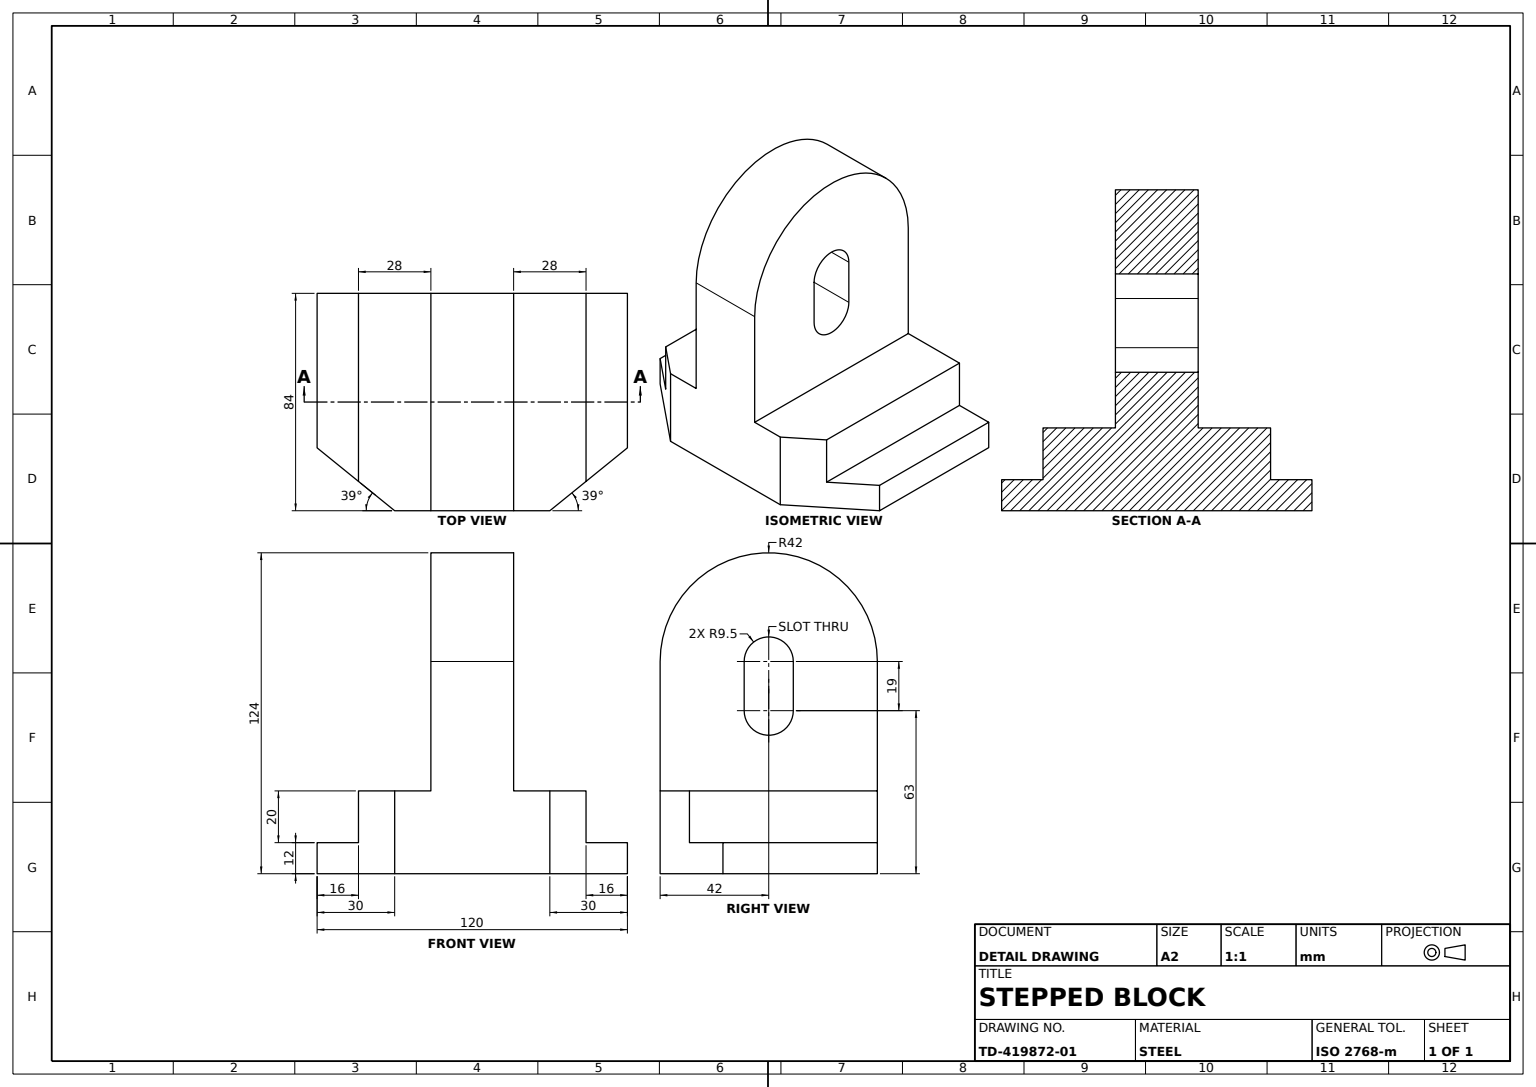
SolidWorks part; units mm, degrees
material "Plain Carbon Steel"
ref_plane "Front Plane" through (0, 0, 0) normal (0, 0, 1) x (1, 0, 0)
ref_plane "Top Plane" through (0, 0, 0) normal (0, 1, 0) x (1, 0, 0)
ref_plane "Right Plane" through (0, 0, 0) normal (1, 0, 0) x (0, 0, -1)
sketch "Bracket Side Profile Sketch" plane through (0, 0, 0) normal (1, 0, 0) x (0, 0, -1)
  line L0 (-60, 0) -> (60, 0)
  line L1 (60, 0) -> (60, 12)
  line L2 (60, 12) -> (44, 12)
  line L3 (44, 12) -> (44, 32)
  line L4 (44, 32) -> (16, 32)
  line L5 (16, 32) -> (16, 124)
  line L6 (0, 0) -> (0, 145.2546) construction
  line L7 (-16, 32) -> (-16, 124)
  line L8 (-44, 32) -> (-16, 32)
  line L9 (-44, 12) -> (-44, 32)
  line L10 (-60, 12) -> (-44, 12)
  line L11 (-60, 0) -> (-60, 12)
  line L12 (-16, 124) -> (16, 124)
  dimension "D1" = 124
  dimension "D2" = 60
  dimension "D3" = 12
  dimension "D4" = 16
  dimension "D5" = 20
  dimension "D6" = 28
extrude "Bracket Body" add sketch "Bracket Side Profile Sketch" along normal mid plane 84
sketch "Upright Profile Cut Sketch" plane through (0, 0, -16) normal (0, 0, -1) x (-1, 0, 0)
  line L0 (42, 0) -> (42, 82) construction
  line L1 (42, 32) -> (42, 124) construction
  line L2 (-42, 82) -> (-42, 124)
  line L3 (-42, 124) -> (42, 124)
  line L4 (42, 124) -> (42, 82)
  arc A0 (42, 82) -> (-42, 82) centre (0, 82) ccw
  line M2 (42, 32) -> (42, 124)
  line M3 (42, 124) -> (-42, 124)
  line M4 (-42, 124) -> (-42, 32)
extrude "Upright Profile Cut" cut sketch "Upright Profile Cut Sketch" against normal blind 40 contours A0 L3 M4 | A0 M2 M3
sketch "Guide Slot Sketch" plane through (0, 0, -16) normal (0, 0, -1) x (-1, 0, 0)
  line L0 (0, 32) -> (0, 124) construction
  line L1 (-42, 32) -> (42, 32) construction
  line L2 (0, 82) -> (0, 63) construction
  line L3 (9.5, 82) -> (9.5, 63)
  line L4 (-9.5, 82) -> (-9.5, 63)
  arc A0 (42, 82) -> (-42, 82) centre (0, 82) ccw construction
  arc A1 (9.5, 82) -> (-9.5, 82) centre (0, 82) ccw
  arc A2 (-9.5, 63) -> (9.5, 63) centre (0, 63) ccw
  point P10 (0, 72.5)
  dimension "D1" = 19
  dimension "D2" = 19
extrude "Guide Slot" cut sketch "Guide Slot Sketch" against normal blind 40
sketch "Angled Corner Cut Sketch 39deg" plane through (0, 32, 0) normal (0, 1, 0) x (1, 0, 0)
  line L0 (0, 0) -> (42, 0) construction
  line L2 (42, 44) -> (42, 16) construction
  line L3 (42, 30) -> (17.7065, 60)
  line L4 (42, 60) -> (-42, 60) construction
  line L5 (17.7065, 60) -> (42, 60)
  line L6 (42, 60) -> (42, 30)
  line L7 (42, -16) -> (42, 16) construction
  line L8 (42, -60) -> (42, -30)
  line L9 (17.7065, -60) -> (42, -60)
  line L10 (42, -30) -> (17.7065, -60)
  dimension "D1" = 39
extrude "Angled Corner Cut 39deg" cut sketch "Angled Corner Cut Sketch 39deg" against normal blind 40
